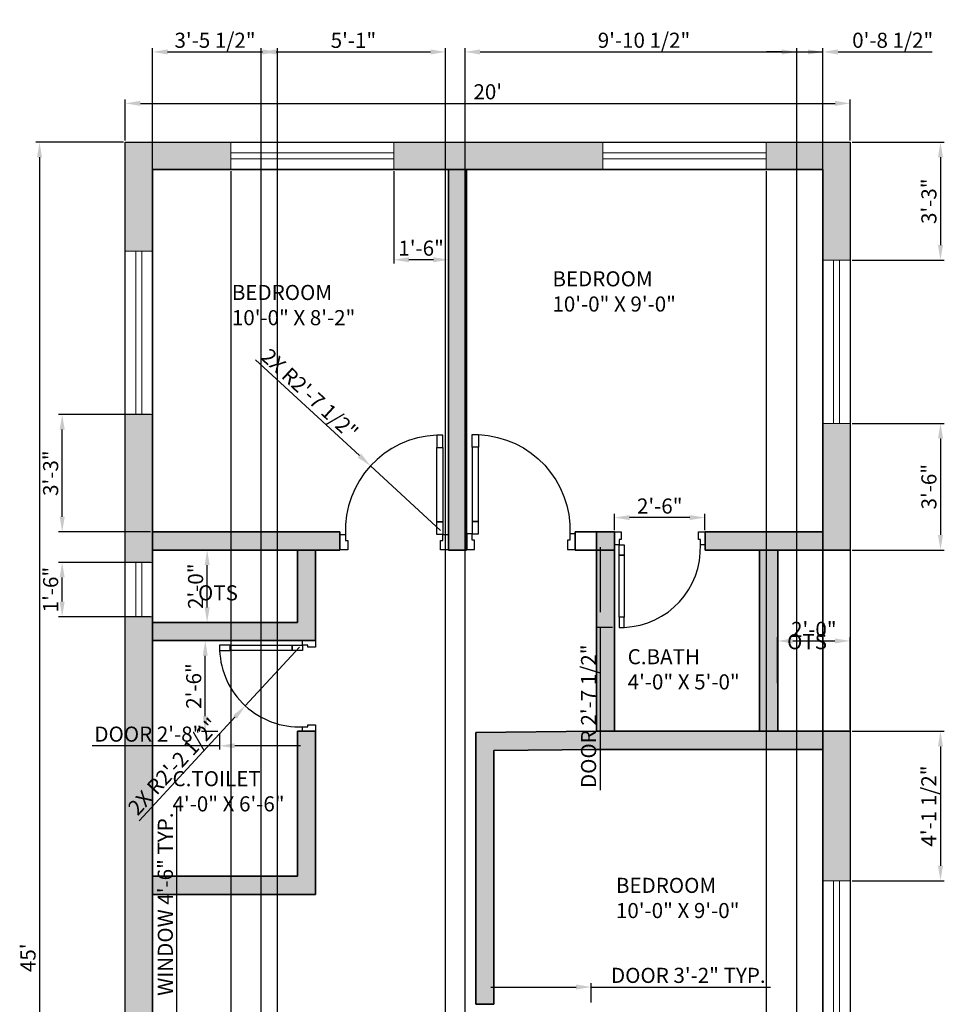
# Model space of a CAD drawing. Units: inches. Extents: x -32 to 277, y -560 to 55.
# Tile 2 of 2: x -32 to 277, y -271 to 55. Entities that reach past the tile are written whole.
import ezdxf

# ---------------------------------------------------------------- set-up
doc = ezdxf.new("R2010")
doc.units = ezdxf.units.IN
for name, color, linetype, lineweight in [('A-ANNO-DIMS', 2, 'Continuous', 18), ('A-AREA-IDEN', 7, 'Continuous', 18), ('A-DOOR', 3, 'Continuous', 25), ('A-GLAZ', 4, 'Continuous', 18), ('A-WALL', 7, 'Continuous', 35), ('A-WALL-PATT', 252, 'Continuous', 13), ('C-PROP', 8, 'Continuous', 25)]:
    doc.layers.add(name, color=color, linetype=linetype, lineweight=lineweight)
doc.styles.get("Standard").update_dxf_attribs({"font": 'arial.ttf'})
doc.dimstyles.new('ISO-25', dxfattribs={"dimtxt": 5, "dimasz": 5, "dimexe": 1.25, "dimexo": 0.625, "dimtad": 1, "dimlunit": 3, "dimtxsty": 'Standard', "dimcen": 2.5, "dimadec": 0, "dimazin": 0, "dimtfac": 1, "dimtmove": 0, "dimatfit": 3, "dimfxl": 1, "dimarcsym": 0})

# ---------------------------------------------------------------- blocks, each defined once
blk = doc.blocks.new('A$C69F834CB')
for points in [[(625, 740), (625, 660), (665, 660), (665, 740)], [(625, 180), (625, 660), (665, 660), (665, 180)], [(625, 100), (625, 180), (665, 180), (665, 100)], [(35, 100), (35, 60), (50, 60), (50, 50), (50, 0), (0, 0), (0, 100)], [(665, 100), (700, 100), (700, 0), (650, 0), (650, 50), (650, 60), (665, 60)]]:
    blk.add_lwpolyline(points, close=True)
blk.add_arc((650, 125), 615.5, 92.32782, 182.32782)
blk = doc.blocks.new('*D2')
at = {"layer": 'A-ANNO-DIMS', "color": 0, "lineweight": -2, "transparency": 16777216}
for p, q in [((2.51, 15.39), (2.51, 28.89)), ((7.51, 27.64), (237.51, 27.64)), ((242.51, 15.39), (242.51, 28.89))]:
    blk.add_line(p, q, dxfattribs=at)
at = {"layer": 'A-ANNO-DIMS', "color": 0, "transparency": 16777216}
for points in [[(7.51, 28.47), (7.51, 26.81), (2.51, 27.64)], [(237.51, 28.47), (237.51, 26.81), (242.51, 27.64)]]:
    blk.add_solid(points, dxfattribs=at)
at = {"layer": 'Defpoints', "color": 0, "transparency": 16777216}
for p in [(242.51, 27.64), (2.51, 14.77), (242.51, 14.77)]:
    blk.add_point(p, dxfattribs=at)
at = {"layer": 'A-ANNO-DIMS', "color": 0, "transparency": 16777216, "insert": (122.51, 30.82), "char_height": 5, "attachment_point": 5}
blk.add_mtext("20'", dxfattribs=at)
blk = doc.blocks.new('*D3')
at = {"layer": 'A-ANNO-DIMS', "color": 0, "lineweight": -2, "transparency": 16777216}
for p, q in [((1.88, 14.77), (-27.13, 14.77)), ((-25.88, 9.77), (-25.88, -520.23)), ((1.88, -525.23), (-27.13, -525.23))]:
    blk.add_line(p, q, dxfattribs=at)
at = {"layer": 'A-ANNO-DIMS', "color": 0, "transparency": 16777216}
for points in [[(-26.72, 9.77), (-25.05, 9.77), (-25.88, 14.77)], [(-26.72, -520.23), (-25.05, -520.23), (-25.88, -525.23)]]:
    blk.add_solid(points, dxfattribs=at)
at = {"layer": 'Defpoints', "color": 0, "transparency": 16777216}
for p in [(2.51, 14.77), (-25.88, -525.23), (2.51, -525.23)]:
    blk.add_point(p, dxfattribs=at)
at = {"layer": 'A-ANNO-DIMS', "color": 0, "transparency": 16777216, "insert": (-29.05, -255.23), "char_height": 5, "attachment_point": 5, "rotation": 90}
blk.add_mtext("45'", dxfattribs=at)
blk = doc.blocks.new('WIN-54IN-9IN-WALL')
for p, q in [((3.5, 0), (3.5, 54)), ((5.5, 0), (5.5, 54))]:
    blk.add_line(p, q)
blk.add_lwpolyline([(9, 54), (9, 0), (0, 0), (0, 54)], close=True)
blk = doc.blocks.new('*D6')
at = {"layer": 'A-ANNO-DIMS', "color": 0, "lineweight": -2, "transparency": 16777216}
for p, q in [((19.61, -274.74), (19.61, -205.22)), ((12.13, -274.74), (20.86, -274.74)), ((19.61, -323.74), (19.61, -279.74)), ((12.13, -328.74), (20.86, -328.74))]:
    blk.add_line(p, q, dxfattribs=at)
at = {"layer": 'A-ANNO-DIMS', "color": 0, "transparency": 16777216}
for points in [[(18.78, -279.74), (20.44, -279.74), (19.61, -274.74)], [(18.78, -323.74), (20.44, -323.74), (19.61, -328.74)]]:
    blk.add_solid(points, dxfattribs=at)
at = {"layer": 'Defpoints', "color": 0, "transparency": 16777216}
for p in [(11.51, -274.74), (19.61, -274.74), (11.51, -328.74)]:
    blk.add_point(p, dxfattribs=at)
at = {"layer": 'A-ANNO-DIMS', "color": 0, "transparency": 16777216, "insert": (16.4, -237.48), "char_height": 5, "attachment_point": 5, "rotation": 90}
blk.add_mtext('WINDOW 4\'-6" TYP.', dxfattribs=at)
blk = doc.blocks.new('*D10')
at = {"layer": 'A-ANNO-DIMS', "color": 0, "lineweight": -2, "transparency": 16777216}
for p, q in [((118.58, -270.01), (118.58, -263.66)), ((156.74, -270.01), (156.74, -263.66)), ((123.58, -264.91), (151.74, -264.91)), ((156.74, -264.91), (216.11, -264.91))]:
    blk.add_line(p, q, dxfattribs=at)
at = {"layer": 'A-ANNO-DIMS', "color": 0, "transparency": 16777216}
for points in [[(123.58, -264.08), (123.58, -265.74), (118.58, -264.91)], [(151.74, -264.08), (151.74, -265.74), (156.74, -264.91)]]:
    blk.add_solid(points, dxfattribs=at)
at = {"layer": 'Defpoints', "color": 0, "transparency": 16777216}
for p in [(156.74, -264.91), (118.58, -270.63), (156.74, -270.63)]:
    blk.add_point(p, dxfattribs=at)
at = {"layer": 'A-ANNO-DIMS', "color": 0, "transparency": 16777216, "insert": (188.92, -261.7), "char_height": 5, "attachment_point": 5}
blk.add_mtext('DOOR 3\'-2" TYP.', dxfattribs=at)
blk = doc.blocks.new('*D12')
at = {"layer": 'A-ANNO-DIMS', "color": 0, "lineweight": -2, "transparency": 16777216}
for p, q in [((33.74, -180.91), (33.74, -186.3)), ((65.51, -180.91), (65.51, -186.3)), ((33.74, -185.05), (-8.44, -185.05)), ((60.51, -185.05), (38.74, -185.05))]:
    blk.add_line(p, q, dxfattribs=at)
at = {"layer": 'A-ANNO-DIMS', "color": 0, "transparency": 16777216}
for points in [[(38.74, -184.21), (38.74, -185.88), (33.74, -185.05)], [(60.51, -184.21), (60.51, -185.88), (65.51, -185.05)]]:
    blk.add_solid(points, dxfattribs=at)
at = {"layer": 'Defpoints', "color": 0, "transparency": 16777216}
for p in [(33.74, -180.28), (65.51, -180.28), (33.74, -185.05)]:
    blk.add_point(p, dxfattribs=at)
at = {"layer": 'A-ANNO-DIMS', "color": 0, "transparency": 16777216, "insert": (10.15, -181.83), "char_height": 5, "attachment_point": 5}
blk.add_mtext('DOOR 2\'-8"', dxfattribs=at)
blk = doc.blocks.new('*D13')
at = {"layer": 'A-ANNO-DIMS', "color": 0, "lineweight": -2, "transparency": 16777216}
for p, q in [((33.12, -150.23), (27.73, -150.23)), ((28.98, -175.28), (28.98, -155.23)), ((33.12, -180.28), (27.73, -180.28))]:
    blk.add_line(p, q, dxfattribs=at)
at = {"layer": 'A-ANNO-DIMS', "color": 0, "transparency": 16777216}
for points in [[(28.15, -155.23), (29.81, -155.23), (28.98, -150.23)], [(28.15, -175.28), (29.81, -175.28), (28.98, -180.28)]]:
    blk.add_solid(points, dxfattribs=at)
at = {"layer": 'Defpoints', "color": 0, "transparency": 16777216}
for p in [(28.98, -150.23), (33.74, -150.23), (33.74, -180.28)]:
    blk.add_point(p, dxfattribs=at)
at = {"layer": 'A-ANNO-DIMS', "color": 0, "transparency": 16777216, "insert": (25.8, -165.26), "char_height": 5, "attachment_point": 5, "rotation": 90}
blk.add_mtext('2\'-6"', dxfattribs=at)
blk = doc.blocks.new('*D14')
at = {"layer": 'A-ANNO-DIMS', "color": 0, "lineweight": -2, "transparency": 16777216}
for p, q in [((163.87, -114.24), (158.51, -114.24)), ((159.76, -119.24), (159.76, -140.85)), ((163.87, -145.85), (158.51, -145.85)), ((159.76, -145.85), (159.76, -199.69))]:
    blk.add_line(p, q, dxfattribs=at)
at = {"layer": 'A-ANNO-DIMS', "color": 0, "transparency": 16777216}
for points in [[(158.92, -119.24), (160.59, -119.24), (159.76, -114.24)], [(158.92, -140.85), (160.59, -140.85), (159.76, -145.85)]]:
    blk.add_solid(points, dxfattribs=at)
at = {"layer": 'Defpoints', "color": 0, "transparency": 16777216}
for p in [(164.5, -114.24), (159.76, -145.85), (164.5, -145.85)]:
    blk.add_point(p, dxfattribs=at)
at = {"layer": 'A-ANNO-DIMS', "color": 0, "transparency": 16777216, "insert": (156.55, -175.27), "char_height": 5, "attachment_point": 5, "rotation": 90}
blk.add_mtext('DOOR 2\'-7 1/2"', dxfattribs=at)
blk = doc.blocks.new('*D15')
at = {"layer": 'A-ANNO-DIMS', "color": 0, "lineweight": -2, "transparency": 16777216}
for p, q in [((164.5, -113.62), (164.5, -108.25)), ((189.4, -109.5), (169.5, -109.5)), ((194.4, -113.62), (194.4, -108.25))]:
    blk.add_line(p, q, dxfattribs=at)
at = {"layer": 'A-ANNO-DIMS', "color": 0, "transparency": 16777216}
for points in [[(169.5, -108.67), (169.5, -110.33), (164.5, -109.5)], [(189.4, -108.67), (189.4, -110.33), (194.4, -109.5)]]:
    blk.add_solid(points, dxfattribs=at)
at = {"layer": 'Defpoints', "color": 0, "transparency": 16777216}
for p in [(164.5, -109.5), (164.5, -114.24), (194.4, -114.24)]:
    blk.add_point(p, dxfattribs=at)
at = {"layer": 'A-ANNO-DIMS', "color": 0, "transparency": 16777216, "insert": (179.45, -106.32), "char_height": 5, "attachment_point": 5}
blk.add_mtext('2\'-6"', dxfattribs=at)
blk = doc.blocks.new('*D18')
at = {"layer": 'A-ANNO-DIMS', "color": 0, "lineweight": -2, "transparency": 16777216}
for p, q in [((11.51, 5.14), (11.51, -556.38)), ((37.4, 5.14), (37.4, -556.38)), ((16.51, -555.13), (32.4, -555.13))]:
    blk.add_line(p, q, dxfattribs=at)
at = {"layer": 'A-ANNO-DIMS', "color": 0, "transparency": 16777216}
for points in [[(16.51, -554.3), (16.51, -555.97), (11.51, -555.13)], [(32.4, -554.3), (32.4, -555.97), (37.4, -555.13)]]:
    blk.add_solid(points, dxfattribs=at)
at = {"layer": 'Defpoints', "color": 0, "transparency": 16777216}
for p in [(11.51, 5.77), (37.4, 5.77), (37.4, -555.13)]:
    blk.add_point(p, dxfattribs=at)
at = {"layer": 'A-ANNO-DIMS', "color": 0, "transparency": 16777216, "insert": (24.45, -552), "char_height": 5, "attachment_point": 5}
blk.add_mtext('2\'-2"', dxfattribs=at)
blk = doc.blocks.new('*D19')
at = {"layer": 'A-ANNO-DIMS', "color": 0, "lineweight": -2, "transparency": 16777216}
for p, q in [((91.4, 5.14), (91.4, -25.38)), ((109.51, 5.14), (109.51, -25.38)), ((104.51, -24.13), (96.4, -24.13))]:
    blk.add_line(p, q, dxfattribs=at)
at = {"layer": 'A-ANNO-DIMS', "color": 0, "transparency": 16777216}
for points in [[(96.4, -23.3), (96.4, -24.97), (91.4, -24.13)], [(104.51, -23.3), (104.51, -24.97), (109.51, -24.13)]]:
    blk.add_solid(points, dxfattribs=at)
at = {"layer": 'Defpoints', "color": 0, "transparency": 16777216}
for p in [(91.4, 5.77), (109.51, 5.77), (91.4, -24.13)]:
    blk.add_point(p, dxfattribs=at)
at = {"layer": 'A-ANNO-DIMS', "color": 0, "transparency": 16777216, "insert": (100.45, -20.95), "char_height": 5, "attachment_point": 5}
blk.add_mtext('1\'-6"', dxfattribs=at)
blk = doc.blocks.new('*D20')
at = {"layer": 'A-ANNO-DIMS', "color": 0, "lineweight": -2, "transparency": 16777216}
for p, q in [((214.66, 5.14), (214.66, -556.38)), ((233.51, 5.14), (233.51, -556.38)), ((219.66, -555.13), (228.51, -555.13))]:
    blk.add_line(p, q, dxfattribs=at)
at = {"layer": 'A-ANNO-DIMS', "color": 0, "transparency": 16777216}
for points in [[(219.66, -554.3), (219.66, -555.97), (214.66, -555.13)], [(228.51, -554.3), (228.51, -555.97), (233.51, -555.13)]]:
    blk.add_solid(points, dxfattribs=at)
at = {"layer": 'Defpoints', "color": 0, "transparency": 16777216}
for p in [(214.66, 5.77), (233.51, 5.77), (233.51, -555.13)]:
    blk.add_point(p, dxfattribs=at)
at = {"layer": 'A-ANNO-DIMS', "color": 0, "transparency": 16777216, "insert": (224.09, -552), "char_height": 5, "attachment_point": 5}
blk.add_mtext('1\'-7"', dxfattribs=at)
blk = doc.blocks.new('*D21')
at = {"layer": 'A-ANNO-DIMS', "color": 0, "lineweight": -2, "transparency": 16777216}
for p, q in [((10.88, -75.35), (-19.64, -75.35)), ((-18.39, -109.23), (-18.39, -80.35)), ((10.88, -114.23), (-19.64, -114.23))]:
    blk.add_line(p, q, dxfattribs=at)
at = {"layer": 'A-ANNO-DIMS', "color": 0, "transparency": 16777216}
for points in [[(-19.22, -80.35), (-17.56, -80.35), (-18.39, -75.35)], [(-19.22, -109.23), (-17.56, -109.23), (-18.39, -114.23)]]:
    blk.add_solid(points, dxfattribs=at)
at = {"layer": 'Defpoints', "color": 0, "transparency": 16777216}
for p in [(-18.39, -75.35), (11.51, -75.35), (11.51, -114.23)]:
    blk.add_point(p, dxfattribs=at)
at = {"layer": 'A-ANNO-DIMS', "color": 0, "transparency": 16777216, "insert": (-21.57, -94.79), "char_height": 5, "attachment_point": 5, "rotation": 90}
blk.add_mtext('3\'-3"', dxfattribs=at)
blk = doc.blocks.new('*D22')
at = {"layer": 'A-ANNO-DIMS', "color": 0, "lineweight": -2, "transparency": 16777216}
for p, q in [((243.13, 14.77), (273.66, 14.77)), ((272.41, 9.77), (272.41, -19.3)), ((243.13, -24.3), (273.66, -24.3))]:
    blk.add_line(p, q, dxfattribs=at)
at = {"layer": 'A-ANNO-DIMS', "color": 0, "transparency": 16777216}
for points in [[(271.58, 9.77), (273.25, 9.77), (272.41, 14.77)], [(271.58, -19.3), (273.25, -19.3), (272.41, -24.3)]]:
    blk.add_solid(points, dxfattribs=at)
at = {"layer": 'Defpoints', "color": 0, "transparency": 16777216}
for p in [(242.51, 14.77), (242.51, -24.3), (272.41, -24.3)]:
    blk.add_point(p, dxfattribs=at)
at = {"layer": 'A-ANNO-DIMS', "color": 0, "transparency": 16777216, "insert": (269.23, -4.77), "char_height": 5, "attachment_point": 5, "rotation": 90}
blk.add_mtext('3\'-3"', dxfattribs=at)
blk = doc.blocks.new('*D23')
at = {"layer": 'A-ANNO-DIMS', "color": 0, "lineweight": -2, "transparency": 16777216}
for p, q in [((243.13, -78.3), (273.66, -78.3)), ((272.41, -83.3), (272.41, -115.23)), ((243.13, -120.23), (273.66, -120.23))]:
    blk.add_line(p, q, dxfattribs=at)
at = {"layer": 'A-ANNO-DIMS', "color": 0, "transparency": 16777216}
for points in [[(271.58, -83.3), (273.25, -83.3), (272.41, -78.3)], [(271.58, -115.23), (273.25, -115.23), (272.41, -120.23)]]:
    blk.add_solid(points, dxfattribs=at)
at = {"layer": 'Defpoints', "color": 0, "transparency": 16777216}
for p in [(242.51, -78.3), (242.51, -120.23), (272.41, -120.23)]:
    blk.add_point(p, dxfattribs=at)
at = {"layer": 'A-ANNO-DIMS', "color": 0, "transparency": 16777216, "insert": (269.23, -99.27), "char_height": 5, "attachment_point": 5, "rotation": 90}
blk.add_mtext('3\'-6"', dxfattribs=at)
blk = doc.blocks.new('*D24')
at = {"layer": 'A-ANNO-DIMS', "color": 0, "lineweight": -2, "transparency": 16777216}
for p, q in [((10.88, -124.33), (-19.64, -124.33)), ((-18.39, -137.33), (-18.39, -129.33)), ((10.88, -142.33), (-19.64, -142.33))]:
    blk.add_line(p, q, dxfattribs=at)
at = {"layer": 'A-ANNO-DIMS', "color": 0, "transparency": 16777216}
for points in [[(-19.22, -129.33), (-17.56, -129.33), (-18.39, -124.33)], [(-19.22, -137.33), (-17.56, -137.33), (-18.39, -142.33)]]:
    blk.add_solid(points, dxfattribs=at)
at = {"layer": 'Defpoints', "color": 0, "transparency": 16777216}
for p in [(-18.39, -124.33), (11.51, -124.33), (11.51, -142.33)]:
    blk.add_point(p, dxfattribs=at)
at = {"layer": 'A-ANNO-DIMS', "color": 0, "transparency": 16777216, "insert": (-21.57, -133.33), "char_height": 5, "attachment_point": 5, "rotation": 90}
blk.add_mtext('1\'-6"', dxfattribs=at)
blk = doc.blocks.new('*D25')
at = {"layer": 'A-ANNO-DIMS', "color": 0, "lineweight": -2, "transparency": 16777216}
for p, q in [((58.88, -120.23), (28.36, -120.23)), ((29.61, -139.23), (29.61, -125.23)), ((58.88, -144.23), (28.36, -144.23))]:
    blk.add_line(p, q, dxfattribs=at)
at = {"layer": 'A-ANNO-DIMS', "color": 0, "transparency": 16777216}
for points in [[(28.78, -125.23), (30.44, -125.23), (29.61, -120.23)], [(28.78, -139.23), (30.44, -139.23), (29.61, -144.23)]]:
    blk.add_solid(points, dxfattribs=at)
at = {"layer": 'Defpoints', "color": 0, "transparency": 16777216}
for p in [(29.61, -120.23), (59.51, -120.23), (59.51, -144.23)]:
    blk.add_point(p, dxfattribs=at)
at = {"layer": 'A-ANNO-DIMS', "color": 0, "transparency": 16777216, "insert": (26.43, -132.23), "char_height": 5, "attachment_point": 5, "rotation": 90}
blk.add_mtext('2\'-0"', dxfattribs=at)
blk = doc.blocks.new('*D26')
at = {"layer": 'A-ANNO-DIMS', "color": 0, "lineweight": -2, "transparency": 16777216}
for p, q in [((218.51, -179.63), (218.48, -149.1)), ((242.51, -179.61), (242.48, -149.08)), ((223.48, -150.35), (237.48, -150.34))]:
    blk.add_line(p, q, dxfattribs=at)
at = {"layer": 'A-ANNO-DIMS', "color": 0, "transparency": 16777216}
for points in [[(223.48, -149.51), (223.48, -151.18), (218.48, -150.35)], [(237.48, -149.5), (237.48, -151.17), (242.48, -150.33)]]:
    blk.add_solid(points, dxfattribs=at)
at = {"layer": 'Defpoints', "color": 0, "transparency": 16777216}
for p in [(242.48, -150.33), (218.51, -180.25), (242.51, -180.23)]:
    blk.add_point(p, dxfattribs=at)
at = {"layer": 'A-ANNO-DIMS', "color": 0, "transparency": 16777216, "insert": (230.48, -147.16), "char_height": 5, "attachment_point": 5, "rotation": 0.0483}
blk.add_mtext('2\'-0"', dxfattribs=at)
blk = doc.blocks.new('*D27')
at = {"layer": 'A-ANNO-DIMS', "color": 0, "lineweight": -2, "transparency": 16777216}
for p, q in [((243.13, -180.23), (273.66, -180.23)), ((272.41, -185.23), (272.41, -224.76)), ((243.13, -229.76), (273.66, -229.76))]:
    blk.add_line(p, q, dxfattribs=at)
at = {"layer": 'A-ANNO-DIMS', "color": 0, "transparency": 16777216}
for points in [[(271.58, -185.23), (273.25, -185.23), (272.41, -180.23)], [(271.58, -224.76), (273.25, -224.76), (272.41, -229.76)]]:
    blk.add_solid(points, dxfattribs=at)
at = {"layer": 'Defpoints', "color": 0, "transparency": 16777216}
for p in [(242.51, -180.23), (242.51, -229.76), (272.41, -229.76)]:
    blk.add_point(p, dxfattribs=at)
at = {"layer": 'A-ANNO-DIMS', "color": 0, "transparency": 16777216, "insert": (269.2, -205), "char_height": 5, "attachment_point": 5, "rotation": 90}
blk.add_mtext('4\'-1 1/2"', dxfattribs=at)
blk = doc.blocks.new('*D38')
at = {"layer": 'A-ANNO-DIMS', "color": 0, "lineweight": -2, "transparency": 16777216}
for p, q in [((47.51, -515.61), (47.51, 45.92)), ((108.57, -515.61), (108.57, 45.92)), ((52.51, 44.67), (103.57, 44.67))]:
    blk.add_line(p, q, dxfattribs=at)
at = {"layer": 'A-ANNO-DIMS', "color": 0, "transparency": 16777216}
for points in [[(52.51, 45.5), (52.51, 43.83), (47.51, 44.67)], [(103.57, 45.5), (103.57, 43.83), (108.57, 44.67)]]:
    blk.add_solid(points, dxfattribs=at)
at = {"layer": 'Defpoints', "color": 0, "transparency": 16777216}
for p in [(108.57, 44.67), (47.51, -516.23), (108.57, -516.23)]:
    blk.add_point(p, dxfattribs=at)
at = {"layer": 'A-ANNO-DIMS', "color": 0, "transparency": 16777216, "insert": (78.04, 47.85), "char_height": 5, "attachment_point": 5}
blk.add_mtext('5\'-1"', dxfattribs=at)
blk = doc.blocks.new('*D39')
at = {"layer": 'A-ANNO-DIMS', "color": 0, "lineweight": -2, "transparency": 16777216}
for p, q in [((114.99, -524.61), (114.99, 45.92)), ((233.51, -524.61), (233.51, 45.92)), ((119.99, 44.67), (228.51, 44.67))]:
    blk.add_line(p, q, dxfattribs=at)
at = {"layer": 'A-ANNO-DIMS', "color": 0, "transparency": 16777216}
for points in [[(119.99, 45.5), (119.99, 43.83), (114.99, 44.67)], [(228.51, 45.5), (228.51, 43.83), (233.51, 44.67)]]:
    blk.add_solid(points, dxfattribs=at)
at = {"layer": 'Defpoints', "color": 0, "transparency": 16777216}
for p in [(233.51, 44.67), (114.99, -525.23), (233.51, -525.23)]:
    blk.add_point(p, dxfattribs=at)
at = {"layer": 'A-ANNO-DIMS', "color": 0, "transparency": 16777216, "insert": (174.25, 47.88), "char_height": 5, "attachment_point": 5}
blk.add_mtext('9\'-10 1/2"', dxfattribs=at)
blk = doc.blocks.new('*D40')
at = {"layer": 'A-ANNO-DIMS', "color": 0, "lineweight": -2, "transparency": 16777216}
for p, q in [((11.51, -437.61), (11.51, 45.92)), ((52.93, -437.61), (52.93, 45.92)), ((16.51, 44.67), (47.93, 44.67))]:
    blk.add_line(p, q, dxfattribs=at)
at = {"layer": 'A-ANNO-DIMS', "color": 0, "transparency": 16777216}
for points in [[(16.51, 45.5), (16.51, 43.83), (11.51, 44.67)], [(47.93, 45.5), (47.93, 43.83), (52.93, 44.67)]]:
    blk.add_solid(points, dxfattribs=at)
at = {"layer": 'Defpoints', "color": 0, "transparency": 16777216}
for p in [(52.93, 44.67), (11.51, -438.23), (52.93, -438.23)]:
    blk.add_point(p, dxfattribs=at)
at = {"layer": 'A-ANNO-DIMS', "color": 0, "transparency": 16777216, "insert": (32.22, 47.88), "char_height": 5, "attachment_point": 5}
blk.add_mtext('3\'-5 1/2"', dxfattribs=at)
blk = doc.blocks.new('*D41')
at = {"layer": 'A-ANNO-DIMS', "color": 0, "lineweight": -2, "transparency": 16777216}
for p, q in [((224.85, -408), (224.85, 45.92)), ((233.51, -408), (233.51, 45.92)), ((219.85, 44.67), (214.85, 44.67)), ((224.85, 44.67), (233.51, 44.67)), ((238.51, 44.67), (269.7, 44.67))]:
    blk.add_line(p, q, dxfattribs=at)
at = {"layer": 'A-ANNO-DIMS', "color": 0, "transparency": 16777216}
for points in [[(219.85, 45.5), (219.85, 43.83), (224.85, 44.67)], [(238.51, 45.5), (238.51, 43.83), (233.51, 44.67)]]:
    blk.add_solid(points, dxfattribs=at)
at = {"layer": 'Defpoints', "color": 0, "transparency": 16777216}
for p in [(233.51, 44.67), (224.85, -408.63), (233.51, -408.63)]:
    blk.add_point(p, dxfattribs=at)
at = {"layer": 'A-ANNO-DIMS', "color": 0, "transparency": 16777216, "insert": (256.6, 47.88), "char_height": 5, "attachment_point": 5}
blk.add_mtext('0\'-8 1/2"', dxfattribs=at)
blk = doc.blocks.new('*D44')
at = {"layer": 'A-ANNO-DIMS', "color": 0, "lineweight": -2, "transparency": 16777216}
for p, q in [((45.62, -57.26), (80.03, -88.98)), ((106.92, -113.78), (83.71, -92.37))]:
    blk.add_line(p, q, dxfattribs=at)
at = {"layer": 'A-ANNO-DIMS', "color": 0, "transparency": 16777216}
blk.add_solid([(80.59, -88.37), (79.46, -89.6), (83.71, -92.37)], dxfattribs=at)
at = {"layer": 'Defpoints', "color": 0, "transparency": 16777216}
for p in [(83.71, -92.37), (106.92, -113.78)]:
    blk.add_point(p, dxfattribs=at)
at = {"layer": 'A-ANNO-DIMS', "color": 0, "transparency": 16777216, "insert": (63.16, -69.07), "char_height": 5, "attachment_point": 5, "rotation": 317.3277}
blk.add_mtext('2X R2\'-7 1/2"', dxfattribs=at)
blk = doc.blocks.new('*D45')
at = {"layer": 'A-ANNO-DIMS', "color": 0, "lineweight": -2, "transparency": 16777216}
for p, q in [((60.14, -152.38), (42.23, -171.8)), ((7.12, -209.89), (38.85, -175.48))]:
    blk.add_line(p, q, dxfattribs=at)
at = {"layer": 'A-ANNO-DIMS', "color": 0, "transparency": 16777216}
blk.add_solid([(38.23, -174.92), (39.46, -176.05), (42.23, -171.8)], dxfattribs=at)
at = {"layer": 'Defpoints', "color": 0, "transparency": 16777216}
for p in [(60.14, -152.38), (42.23, -171.8)]:
    blk.add_point(p, dxfattribs=at)
at = {"layer": 'A-ANNO-DIMS', "color": 0, "transparency": 16777216, "insert": (18.93, -192.35), "char_height": 5, "attachment_point": 5, "rotation": 47.3277}
blk.add_mtext('2X R2\'-2 1/2"', dxfattribs=at)

msp = doc.modelspace()

# ---------------------------------------------------------------- hatches: boundary and pattern name
at = {"layer": 'A-WALL-PATT'}
h = msp.add_hatch(color=256, dxfattribs=at)
h.dxf.hatch_style = 1
h.paths.add_polyline_path([(11.509, 5.768), (37.398, 5.768), (37.398, 14.768), (2.509, 14.768), (2.509, -21.347), (11.509, -21.347)])
h.paths.add_polyline_path([(160.664, 14.768), (91.398, 14.768), (91.398, 5.768), (160.664, 5.768)])
h.paths.add_polyline_path([(115.509, 5.768), (109.509, 5.768), (109.509, -120.232), (115.509, -120.232)])
h.paths.add_polyline_path([(242.509, 14.768), (214.664, 14.768), (214.664, 5.768), (233.509, 5.768), (233.509, -24.301), (242.509, -24.301)])
h.paths.add_polyline_path([(242.509, -78.301), (233.509, -78.301), (233.509, -114.232), (194.509, -114.232), (194.509, -120.232), (233.509, -120.232), (242.509, -120.232)])
h.paths.add_polyline_path([(73.509, -114.232), (11.509, -114.232), (11.509, -120.232), (73.509, -120.232)])
h.paths.add_polyline_path([(11.509, -75.347), (2.509, -75.347), (2.509, -124.333), (11.509, -124.333)])
h = msp.add_hatch(color=256, dxfattribs=at)
h.dxf.hatch_style = 1
h.paths.add_polyline_path([(218.509, -120.232), (212.509, -120.232), (212.509, -180.252), (218.509, -180.252)])
h.paths.add_polyline_path([(164.509, -120.232), (158.509, -120.232), (158.509, -180.252), (164.509, -180.252)])
h.paths.add_polyline_path([(164.499, -114.232), (158.509, -114.232), (158.509, -120.232), (164.509, -120.232), (164.509, -118.512), (164.499, -118.512)])
h.paths.add_polyline_path([(65.509, -120.232), (59.509, -120.232), (59.509, -144.232), (11.509, -144.232), (11.509, -150.232), (59.509, -150.232), (65.509, -150.232)])
h.paths.add_polyline_path([(65.509, -180.281), (61.216, -180.281), (59.509, -180.232), (59.509, -228.232), (11.509, -228.232), (11.509, -234.232), (65.509, -234.232)])
h.paths.add_polyline_path([(11.509, -142.333), (2.509, -142.333), (2.509, -274.742), (11.509, -274.742)])
h = msp.add_hatch(color=256, dxfattribs=at)
h.dxf.hatch_style = 1
h.paths.add_polyline_path([(242.509, -180.232), (218.509, -180.252), (158.476, -180.252), (118.521, -180.696), (118.521, -186.63), (118.521, -270.63), (124.521, -270.63), (124.521, -186.63), (158.509, -186.252), (218.509, -186.252), (233.509, -186.24), (233.509, -229.761), (242.509, -229.761)])
h.paths.add_polyline_path([(242.509, -283.761), (233.509, -283.761), (233.509, -336.433), (242.509, -336.433)])
h.paths.add_polyline_path([(233.509, -306.63), (123.737, -306.63), (123.737, -306.725), (118.58, -306.725), (112.521, -306.63), (112.521, -312.63), (233.509, -312.63)])
h.paths.add_polyline_path([(11.509, -328.742), (2.509, -328.742), (2.509, -388.159), (11.509, -388.159)])
h.paths.add_polyline_path([(76.975, -354.577), (11.509, -354.577), (11.509, -360.577), (76.975, -360.577)])
h.paths.add_polyline_path([(118.521, -336.63), (112.521, -336.63), (112.521, -381.532), (118.521, -381.532)])
h.paths.add_polyline_path([(242.509, -390.433), (233.509, -390.433), (233.509, -516.232), (233.509, -525.232), (242.509, -525.232)])
h.paths.add_polyline_path([(233.509, -408.63), (224.849, -408.63), (224.849, -414.63), (233.509, -414.63)])
h.paths.add_polyline_path([(170.849, -408.63), (160.521, -408.63), (160.521, -414.63), (170.849, -414.63)])
h.paths.add_polyline_path([(118.521, -438.232), (118.521, -435.532), (112.521, -435.532), (112.521, -438.232), (106.925, -438.232), (106.925, -444.232), (113.551, -444.232), (118.521, -444.232)])
h.paths.add_polyline_path([(52.925, -438.232), (11.509, -438.232), (11.509, -444.232), (52.925, -444.232)], flags=17)
h.paths.add_polyline_path([(11.509, -444.232), (11.509, -422.159), (2.509, -422.159), (2.509, -525.232), (114.994, -525.232), (114.994, -516.232), (11.509, -516.232)])

# ---------------------------------------------------------------- linework, layer by layer
at = {"layer": 'A-GLAZ'}
for p, q in [((6.009, -124.333), (6.009, -142.333)), ((8.009, -124.333), (8.009, -142.333))]:
    msp.add_line(p, q, dxfattribs=at)
msp.add_lwpolyline([(2.509, -124.333), (11.509, -124.333), (11.509, -142.333), (2.509, -142.333)], close=True, dxfattribs=at)
at = {"layer": 'A-WALL'}
for p, q in [((11.509, 5.768), (233.509, 5.768)), ((11.509, -444.232), (11.509, 5.768)), ((109.509, -120.232), (109.509, 5.768)), ((115.509, -120.232), (115.509, 5.768)), ((233.509, 5.768), (233.509, -114.232)), ((11.509, -114.232), (73.509, -114.232)), ((73.509, -114.232), (73.509, -120.232)), ((151.509, -114.232), (164.509, -114.232)), ((151.509, -114.232), (151.509, -120.232)), ((158.509, -120.232), (158.509, -114.232)), ((164.509, -120.232), (164.509, -114.232)), ((194.509, -120.232), (194.509, -114.232)), ((194.509, -114.232), (233.509, -114.232)), ((11.509, -120.232), (73.509, -120.232)), ((59.509, -144.232), (59.509, -120.232)), ((65.509, -150.232), (65.509, -120.232)), ((109.509, -120.232), (115.509, -120.232)), ((151.509, -120.232), (164.509, -120.232)), ((158.509, -180.252), (158.509, -120.232)), ((164.509, -180.252), (164.509, -120.232)), ((194.509, -120.232), (233.509, -120.232)), ((212.509, -180.252), (212.509, -120.232)), ((218.509, -180.252), (218.509, -120.232)), ((233.509, -120.232), (242.509, -120.232)), ((11.509, -144.232), (59.509, -144.232)), ((11.509, -150.232), (59.509, -150.232)), ((59.509, -150.232), (65.509, -150.232)), ((242.509, -155.478), (242.509, -155.478)), ((59.509, -228.232), (59.509, -180.232)), ((59.509, -180.232), (65.509, -180.232)), ((65.509, -234.232), (65.509, -180.232)), ((118.521, -180.696), (158.442, -180.253)), ((118.521, -186.63), (118.521, -180.696)), ((218.509, -180.252), (158.509, -180.252)), ((242.509, -180.232), (218.509, -180.252)), ((118.521, -186.63), (118.521, -270.63)), ((124.521, -186.63), (158.509, -186.252)), ((124.521, -186.63), (124.521, -270.63)), ((218.509, -186.252), (158.509, -186.252)), ((233.509, -186.24), (218.514, -186.252)), ((233.509, -186.24), (233.509, -516.232)), ((242.514, -186.232), (242.509, -186.232)), ((11.509, -228.232), (59.509, -228.232)), ((11.509, -234.232), (65.509, -234.232)), ((124.521, -270.63), (118.521, -270.63))]:
    msp.add_line(p, q, dxfattribs=at)
at = {"layer": 'C-PROP'}
msp.add_lwpolyline([(2.509, 14.768), (242.509, 14.768), (242.509, -525.232), (2.509, -525.232)], close=True, dxfattribs=at)

# ---------------------------------------------------------------- block references
at = {"layer": 'A-DOOR'}
for p, xscale, yscale, zscale in [((73.576, -120.19), 0.0513040572500651, 0.0513040572500651, 0.0513040572500651), ((151.532, -120.032), -0.0513481873511358, 0.0513481873511358, 0.0513481873511358)]:
    msp.add_blockref('A$C69F834CB', p, dxfattribs=dict(at, xscale=xscale, yscale=yscale, zscale=zscale))
for p, xscale, yscale, zscale, rotation in [((194.399, -114.24), 0.0427139791089293, 0.0427139791089293, 0.0427139791089293, 180), ((65.509, -180.281), 0.0429266772448446, 0.0429266772448446, 0.0429266772448446, 90.00000000000003)]:
    msp.add_blockref('A$C69F834CB', p, dxfattribs=dict(at, xscale=xscale, yscale=yscale, zscale=zscale, rotation=rotation))
at = {"layer": 'A-GLAZ'}
for p, rotation in [((91.397, 5.768), 90), ((214.664, 5.768), 90.00000000000003)]:
    msp.add_blockref('WIN-54IN-9IN-WALL', p, dxfattribs=dict(at, rotation=rotation))
for p in [(2.509, -75.347), (233.509, -78.3), (233.509, -283.761)]:
    msp.add_blockref('WIN-54IN-9IN-WALL', p, dxfattribs=at)

# ---------------------------------------------------------------- texts
at = {"layer": 'A-AREA-IDEN', "char_height": 5, "attachment_point": 1}
for s, width, insert in [('BEDROOM\\P10\'-0" X 9\'-0"', 54.4563, (143.931, -27.955)), ('BEDROOM\\P10\'-0" X 8\'-2"', 47.85934, (37.789, -32.469)), ('OTS', 28.41798, (26.591, -131.914)), ('OTS', 13.10458, (221.632, -148.086)), ('C.BATH\\P4\'-0" X 5\'-0"', 39.73761, (168.834, -153.058)), ('C.TOILET\\P4\'-0" X 6\'-6"', 40.09565, (18.141, -193.438)), ('BEDROOM\\P10\'-0" X 9\'-0"', 52.63609, (164.955, -228.76))]:
    msp.add_mtext_dynamic_manual_height_columns(s, width=width, gutter_width=12.5, heights=[0], dxfattribs=dict(at, insert=insert))

# ---------------------------------------------------------------- dimensions: what is measured, and where the dimension line sits
at = {"layer": 'A-ANNO-DIMS'}
for base, p1, p2, override, picture, middle in [((52.925, 44.668), (11.509, -438.232), (52.925, -438.232), {"dimdec": 1, "dimlfac": 1, "dimrnd": 0, "dimzin": 1, "dimdsep": 46, "dimlunit": 4, "dimfrac": 2}, '*D40', (32.217, 47.88)), ((233.509, 44.668), (114.994, -525.232), (233.509, -525.232), {"dimdec": 1, "dimlfac": 1, "dimrnd": 0, "dimzin": 1, "dimdsep": 46, "dimlunit": 4, "dimfrac": 2}, '*D39', (174.252, 47.878)), ((233.509, 44.668), (224.849, -408.63), (233.509, -408.63), {"dimdec": 1, "dimlfac": 1, "dimrnd": 0, "dimzin": 1, "dimdsep": 46, "dimlunit": 4, "dimfrac": 2}, '*D41', (256.605, 47.878)), ((108.573, 44.668), (47.509, -516.232), (108.573, -516.232), {"dimdec": 1, "dimlfac": 1, "dimrnd": 0, "dimzin": 1, "dimdsep": 46, "dimlunit": 4, "dimfrac": 2}, '*D38', (78.041, 47.846)), ((242.509, 27.641), (2.509, 14.768), (242.509, 14.768), {"dimclrd": 0, "dimclre": 0, "dimclrt": 0}, '*D2', (122.509, 30.819)), ((37.398, -555.132), (11.509, 5.768), (37.398, 5.768), {"dimdec": 1, "dimlfac": 1, "dimrnd": 0, "dimzin": 1, "dimdsep": 46, "dimlunit": 4, "dimfrac": 2}, '*D18', (24.453, -551.997)), ((233.509, -555.132), (214.664, 5.768), (233.509, 5.768), {"dimdec": 1, "dimlfac": 1, "dimrnd": 0, "dimzin": 1, "dimdsep": 46, "dimlunit": 4, "dimfrac": 2}, '*D20', (224.087, -551.997))]:
    dim = msp.add_linear_dim(base=base, p1=p1, p2=p2, dimstyle='ISO-25', override=override, dxfattribs=at)
    dim.commit()
    dim.dimension.update_dxf_attribs({"geometry": picture, "text_midpoint": middle})
for base, p1, p2, angle, override, picture, middle in [((-25.883, -525.232), (2.509, 14.768), (2.509, -525.232), 90, {"dimclrd": 0, "dimclre": 0, "dimclrt": 0}, '*D3', (-29.051, -255.232)), ((272.414, -24.301), (242.509, 14.768), (242.509, -24.301), 90, {"dimdec": 1, "dimlfac": 1, "dimrnd": 0, "dimzin": 1, "dimdsep": 46, "dimlunit": 4, "dimfrac": 2}, '*D22', (269.234, -4.766)), ((91.398, -24.132), (109.509, 5.768), (91.398, 5.768), 180, {"dimdec": 1, "dimlfac": 1, "dimrnd": 0, "dimzin": 1, "dimdsep": 46, "dimlunit": 4, "dimfrac": 2}, '*D19', (100.453, -20.954)), ((-18.391, -75.347), (11.509, -114.232), (11.509, -75.347), 90, {"dimdec": 1, "dimlfac": 1, "dimrnd": 0, "dimzin": 1, "dimdsep": 46, "dimlunit": 4, "dimfrac": 2}, '*D21', (-21.571, -94.79)), ((272.414, -120.232), (242.509, -78.301), (242.509, -120.232), 90, {"dimdec": 1, "dimlfac": 1, "dimrnd": 0, "dimzin": 1, "dimdsep": 46, "dimlunit": 4, "dimfrac": 2}, '*D23', (269.234, -99.266)), ((164.499, -109.499), (194.399, -114.24), (164.499, -114.24), 180, {"dimdec": 1, "dimlfac": 1, "dimrnd": 0, "dimzin": 1, "dimdsep": 46, "dimlunit": 4, "dimfrac": 2}, '*D15', (179.449, -106.321)), ((29.609, -120.232), (59.509, -144.232), (59.509, -120.232), 90, {"dimdec": 1, "dimlfac": 1, "dimrnd": 0, "dimzin": 1, "dimdsep": 46, "dimlunit": 4, "dimfrac": 2}, '*D25', (26.431, -132.232)), ((-18.391, -124.333), (11.509, -142.333), (11.509, -124.333), 90, {"dimdec": 1, "dimlfac": 1, "dimrnd": 0, "dimzin": 1, "dimdsep": 46, "dimlunit": 4, "dimfrac": 2}, '*D24', (-21.569, -133.333)), ((242.484, -150.332), (218.509, -180.252), (242.509, -180.232), 0.04833, {"dimdec": 1, "dimlfac": 1, "dimrnd": 0, "dimzin": 1, "dimdsep": 46, "dimlunit": 4, "dimfrac": 2}, '*D26', (230.481, -147.164)), ((28.978, -150.232), (33.743, -180.281), (33.743, -150.232), 90, {"dimdec": 1, "dimlfac": 1, "dimrnd": 0, "dimzin": 1, "dimdsep": 46, "dimlunit": 4, "dimfrac": 2}, '*D13', (25.8, -165.256)), ((272.414, -229.761), (242.509, -180.232), (242.509, -229.761), 90, {"dimdec": 1, "dimlfac": 1, "dimrnd": 0, "dimzin": 1, "dimdsep": 46, "dimlunit": 4, "dimfrac": 2}, '*D27', (269.204, -204.997))]:
    dim = msp.add_linear_dim(base=base, p1=p1, p2=p2, angle=angle, dimstyle='ISO-25', override=override, dxfattribs=at)
    dim.commit()
    dim.dimension.update_dxf_attribs({"geometry": picture, "text_midpoint": middle})
for center, mpoint, picture, middle in [((106.924, -113.777), (83.706, -92.373), '*D44', (63.161, -69.066)), ((60.143, -152.378), (42.234, -171.805), '*D45', (18.928, -192.35))]:
    dim = msp.add_radius_dim(center=center, mpoint=mpoint, text='2X <>', dimstyle='ISO-25', override={"dimdec": 1, "dimlfac": 1, "dimrnd": 0, "dimzin": 1, "dimdsep": 46, "dimlunit": 4, "dimfrac": 2}, dxfattribs=at)
    dim.commit()
    dim.dimension.update_dxf_attribs({"geometry": picture, "text_midpoint": middle})
for base, p1, p2, angle, text, picture, middle in [((159.758, -145.849), (164.499, -114.24), (164.499, -145.849), 270, 'DOOR <>', '*D14', (156.546, -175.268)), ((33.743, -185.045), (65.509, -180.281), (33.743, -180.281), 180, 'DOOR <>', '*D12', (10.149, -181.833)), ((19.609, -274.742), (11.509, -328.742), (11.509, -274.742), 90, 'WINDOW <> TYP.', '*D6', (16.397, -237.482))]:
    dim = msp.add_linear_dim(base=base, p1=p1, p2=p2, angle=angle, text=text, dimstyle='ISO-25', override={"dimdec": 1, "dimlfac": 1, "dimrnd": 0, "dimzin": 1, "dimdsep": 46, "dimlunit": 4, "dimfrac": 2}, dxfattribs=at)
    dim.commit()
    dim.dimension.update_dxf_attribs({"geometry": picture, "text_midpoint": middle})
dim = msp.add_linear_dim(base=(156.736, -264.909), p1=(118.58, -270.632), p2=(156.736, -270.632), text='DOOR <> TYP.', dimstyle='ISO-25', override={"dimdec": 1, "dimlfac": 1, "dimrnd": 0, "dimzin": 1, "dimdsep": 46, "dimlunit": 4, "dimfrac": 2}, dxfattribs=at)
dim.commit()
dim.dimension.update_dxf_attribs({"geometry": '*D10', "text_midpoint": (188.923, -261.695)})

doc.saveas('drawing.dxf')
